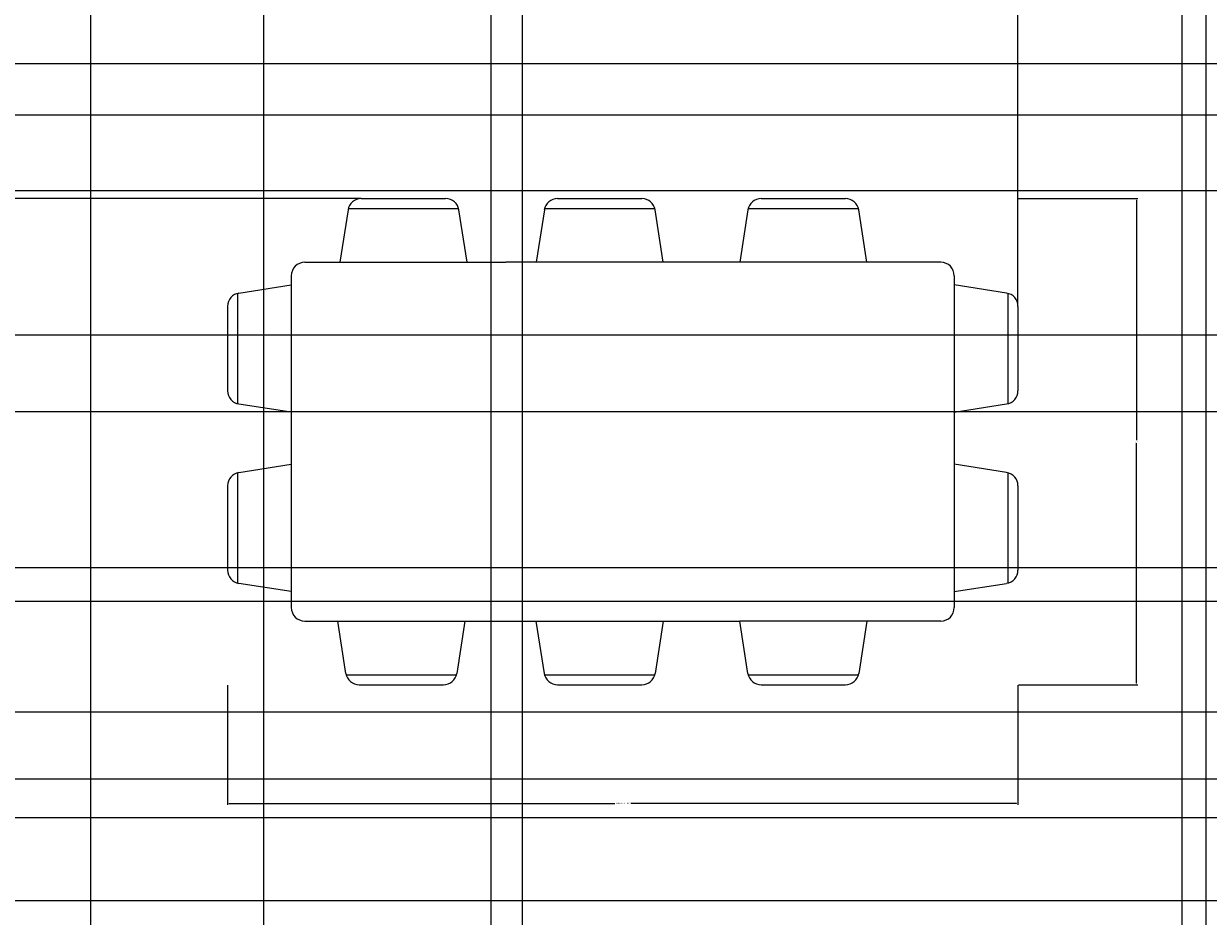
# Model space of a CAD drawing. Units: inches. Extents: x 1531 to 2263, y 2711 to 3216.
# Tile 8 of 12: x 1925 to 2076, y 2901 to 3015. Entities that reach past the tile are written whole.
import ezdxf

# ---------------------------------------------------------------- set-up
doc = ezdxf.new("R2010")
doc.units = ezdxf.units.IN
doc.layers.add('A-ANNO-DIMS', color=2, linetype='Continuous', lineweight=18)
doc.layers.add('A-FURN', color=8, linetype='Continuous', lineweight=18)
doc.styles.get("Standard").update_dxf_attribs({"font": 'arial.ttf'})
doc.dimstyles.get("Standard").update_dxf_attribs({"dimtxt": 0.18, "dimasz": 0.18, "dimexe": 0.18, "dimexo": 0.0625, "dimgap": 0.09, "dimtad": 0, "dimtih": 1, "dimtoh": 1, "dimdec": 4, "dimzin": 0, "dimdsep": 46, "dimtxsty": 'Standard', "dimcen": 0.09, "dimadec": 0, "dimazin": 0, "dimtfac": 1, "dimtdec": 4, "dimtofl": 0, "dimtmove": 0, "dimatfit": 3, "dimfxl": 1, "dimtolj": 1, "dimtzin": 0, "dimarcsym": 0})

# ---------------------------------------------------------------- blocks, each defined once
blk = doc.blocks.new('Dining Set - 36 x 72 in.')
for p, q in [((-27.5, -40.45), (-11.03, -40.45)), ((-25.56, -38.95), (-12.98, -38.95)), ((1.77, -40.45), (18.24, -40.45)), ((3.71, -38.95), (16.29, -38.95)), ((32.13, -40.45), (48.6, -40.45)), ((34.07, -38.95), (46.65, -38.95)), ((-27.53, -40.64), (-28.75, -48.45)), ((-9.78, -48.45), (-11.01, -40.64)), ((1.74, -40.64), (0.52, -48.45)), ((19.48, -48.45), (18.26, -40.64)), ((32.09, -40.64), (30.87, -48.45)), ((49.84, -48.45), (48.62, -40.64)), ((-34, -48.45), (-4, -48.45)), ((26.36, -48.45), (-4, -48.45)), ((60.87, -48.45), (26.36, -48.45)), ((49.84, -48.44), (30.87, -48.44)), ((-36, -50.45), (-36, -75.18)), ((62.87, -50.45), (62.87, -75.18)), ((-43.81, -53.04), (-36, -51.82)), ((70.68, -53.04), (62.87, -51.82)), ((-44, -53.07), (-44, -69.54)), ((70.87, -53.07), (70.87, -69.54)), ((-45.5, -55.01), (-45.5, -67.59)), ((72.37, -55.01), (72.37, -67.59)), ((-36, -70.79), (-43.81, -69.57)), ((62.87, -70.79), (70.68, -69.56)), ((-36, -75.18), (-36, -99.92)), ((62.87, -75.18), (62.87, -99.92)), ((-43.81, -79.77), (-36, -78.55)), ((70.68, -79.77), (62.87, -78.55)), ((-44, -79.81), (-44, -96.28)), ((70.87, -79.81), (70.87, -96.28)), ((-45.5, -81.75), (-45.5, -94.33)), ((72.37, -81.75), (72.37, -94.32)), ((-36, -97.52), (-43.81, -96.3)), ((62.87, -97.52), (70.68, -96.3)), ((-34, -101.92), (-4, -101.92)), ((-27.85, -109.73), (-29.07, -101.92)), ((-10.11, -101.92), (-11.33, -109.73)), ((-4, -101.92), (26.36, -101.92)), ((1.74, -109.73), (0.52, -101.92)), ((19.48, -101.92), (18.26, -109.73)), ((26.36, -101.92), (30.87, -101.92)), ((60.87, -101.92), (30.87, -101.92)), ((32.09, -109.73), (30.87, -101.92)), ((49.84, -101.92), (48.62, -109.73)), ((-27.82, -109.92), (-11.35, -109.92)), ((1.77, -109.92), (18.24, -109.92)), ((32.13, -109.92), (48.6, -109.92)), ((-25.88, -111.42), (-13.3, -111.42)), ((3.71, -111.42), (16.29, -111.42)), ((34.07, -111.42), (46.65, -111.42))]:
    blk.add_line(p, q)
for centre, start, end in [((-25.56, -40.95), 90, 171.1198), ((-12.98, -40.95), 8.881, 90), ((3.71, -40.95), 90, 171.1198), ((16.29, -40.95), 8.881, 90), ((34.07, -40.95), 90, 171.1198), ((46.65, -40.95), 8.881, 90), ((-34, -50.45), 90, 180), ((60.87, -50.45), 0, 90), ((-43.5, -55.01), 98.8806, 180), ((70.37, -55.01), 0, 81.1194), ((-43.5, -67.59), 180, 261.1194), ((70.37, -67.59), 278.8806, 0), ((-43.5, -81.75), 98.8806, 180), ((70.37, -81.75), 0, 81.1194), ((-43.5, -94.33), 180, 261.1194), ((70.37, -94.32), 278.8806, 0), ((-34, -99.92), 180, 270), ((60.87, -99.92), 270, 0), ((-25.88, -109.42), 188.8802, 270), ((-13.3, -109.42), 270, 351.1191), ((3.71, -109.42), 188.8802, 270), ((16.29, -109.42), 270, 351.1191), ((34.07, -109.42), 188.8802, 270), ((46.65, -109.42), 270, 351.1191)]:
    blk.add_arc(centre, 2, start, end)
blk = doc.blocks.new('*D52')
at = {"layer": 'A-ANNO-DIMS', "color": 0, "lineweight": -2, "transparency": 16777216}
for p, q in [((1951.34, 2930.78), (1951.34, 2915.57)), ((2052, 2930.78), (2052, 2915.57)), ((1951.52, 2915.75), (2000.65, 2915.75)), ((2051.82, 2915.75), (2002.69, 2915.75))]:
    blk.add_line(p, q, dxfattribs=at)
at = {"layer": 'A-ANNO-DIMS', "color": 0, "transparency": 16777216}
for points in [[(1951.52, 2915.78), (1951.52, 2915.72), (1951.34, 2915.75)], [(2051.82, 2915.78), (2051.82, 2915.72), (2052, 2915.75)]]:
    blk.add_solid(points, dxfattribs=at)
at = {"layer": 'Defpoints', "color": 0, "transparency": 16777216}
for p in [(1951.34, 2930.85), (2052, 2930.85), (2052, 2915.75)]:
    blk.add_point(p, dxfattribs=at)
at = {"layer": 'A-ANNO-DIMS', "color": 0, "transparency": 16777216, "insert": (2001.67, 2915.75), "char_height": 0.18, "attachment_point": 5}
blk.add_mtext('\\A1;DINING SET 101', dxfattribs=at)
blk = doc.blocks.new('*D53')
at = {"layer": 'A-ANNO-DIMS', "color": 0, "lineweight": -2, "transparency": 16777216}
for p, q in [((2052.06, 2992.73), (2067.28, 2992.73)), ((2067.1, 2992.55), (2067.1, 2961.97)), ((2067.1, 2931.03), (2067.1, 2961.61)), ((2052.06, 2930.85), (2067.28, 2930.85))]:
    blk.add_line(p, q, dxfattribs=at)
at = {"layer": 'A-ANNO-DIMS', "color": 0, "transparency": 16777216}
for points in [[(2067.07, 2992.55), (2067.13, 2992.55), (2067.1, 2992.73)], [(2067.07, 2931.03), (2067.13, 2931.03), (2067.1, 2930.85)]]:
    blk.add_solid(points, dxfattribs=at)
at = {"layer": 'Defpoints', "color": 0, "transparency": 16777216}
for p in [(2052, 2992.73), (2067.1, 2992.73), (2052, 2930.85)]:
    blk.add_point(p, dxfattribs=at)
at = {"layer": 'A-ANNO-DIMS', "color": 0, "transparency": 16777216, "insert": (2067.1, 2961.79), "char_height": 0.18, "attachment_point": 5}
blk.add_mtext('\\A1;62', dxfattribs=at)
blk = doc.blocks.new('*D60')
at = {"layer": 'A-ANNO-DIMS', "color": 0, "lineweight": -2, "transparency": 16777216}
for p, q in [((1899.91, 3097.79), (1899.91, 2711.06)), ((1955.91, 3097.81), (1955.91, 2711.06)), ((1900.09, 2711.24), (1927.69, 2711.24)), ((1955.73, 2711.24), (1928.13, 2711.24))]:
    blk.add_line(p, q, dxfattribs=at)
at = {"layer": 'A-ANNO-DIMS', "color": 0, "transparency": 16777216}
for points in [[(1900.09, 2711.27), (1900.09, 2711.21), (1899.91, 2711.24)], [(1955.73, 2711.27), (1955.73, 2711.21), (1955.91, 2711.24)]]:
    blk.add_solid(points, dxfattribs=at)
at = {"layer": 'Defpoints', "color": 0, "transparency": 16777216}
for p in [(1899.91, 3097.85), (1955.91, 3097.88), (1955.91, 2711.24)]:
    blk.add_point(p, dxfattribs=at)
at = {"layer": 'A-ANNO-DIMS', "color": 0, "transparency": 16777216, "insert": (1927.91, 2711.24), "char_height": 0.18, "attachment_point": 5}
blk.add_mtext('\\A1;56', dxfattribs=at)
blk = doc.blocks.new('*D71')
at = {"layer": 'A-ANNO-DIMS', "color": 0, "lineweight": -2, "transparency": 16777216}
for p, q in [((1933.91, 2891.93), (1933.91, 3216.47)), ((1984.91, 2891.95), (1984.91, 3216.47)), ((1934.09, 3216.29), (1959.21, 3216.29)), ((1984.73, 3216.29), (1959.61, 3216.29))]:
    blk.add_line(p, q, dxfattribs=at)
at = {"layer": 'A-ANNO-DIMS', "color": 0, "transparency": 16777216}
for points in [[(1934.09, 3216.32), (1934.09, 3216.26), (1933.91, 3216.29)], [(1984.73, 3216.32), (1984.73, 3216.26), (1984.91, 3216.29)]]:
    blk.add_solid(points, dxfattribs=at)
at = {"layer": 'Defpoints', "color": 0, "transparency": 16777216}
for p in [(1984.91, 3216.29), (1933.91, 2891.87), (1984.91, 2891.89)]:
    blk.add_point(p, dxfattribs=at)
at = {"layer": 'A-ANNO-DIMS', "color": 0, "transparency": 16777216, "insert": (1959.41, 3216.29), "char_height": 0.18, "attachment_point": 5}
blk.add_mtext('\\A1;51', dxfattribs=at)
blk = doc.blocks.new('*D77')
at = {"layer": 'A-ANNO-DIMS', "color": 0, "lineweight": -2, "transparency": 16777216}
for p, q in [((2094.81, 2975.33), (1531.04, 2975.33)), ((1531.22, 2975.15), (1531.22, 2939.52)), ((1531.22, 2903.53), (1531.22, 2939.16)), ((2094.81, 2903.35), (1531.04, 2903.35))]:
    blk.add_line(p, q, dxfattribs=at)
at = {"layer": 'A-ANNO-DIMS', "color": 0, "transparency": 16777216}
for points in [[(1531.19, 2975.15), (1531.25, 2975.15), (1531.22, 2975.33)], [(1531.19, 2903.53), (1531.25, 2903.53), (1531.22, 2903.35)]]:
    blk.add_solid(points, dxfattribs=at)
at = {"layer": 'Defpoints', "color": 0, "transparency": 16777216}
for p in [(2094.87, 2975.33), (1531.22, 2903.35), (2094.87, 2903.35)]:
    blk.add_point(p, dxfattribs=at)
at = {"layer": 'A-ANNO-DIMS', "color": 0, "transparency": 16777216, "insert": (1531.22, 2939.34), "char_height": 0.18, "attachment_point": 5}
blk.add_mtext('\\A1;71.98', dxfattribs=at)
blk = doc.blocks.new('*D79')
at = {"layer": 'A-ANNO-DIMS', "color": 0, "lineweight": -2, "transparency": 16777216}
for p, q in [((1988.91, 2807.93), (1988.91, 3216.47)), ((2072.91, 2807.93), (2072.91, 3216.47)), ((1989.09, 3216.29), (2030.69, 3216.29)), ((2072.73, 3216.29), (2031.13, 3216.29))]:
    blk.add_line(p, q, dxfattribs=at)
at = {"layer": 'A-ANNO-DIMS', "color": 0, "transparency": 16777216}
for points in [[(1989.09, 3216.32), (1989.09, 3216.26), (1988.91, 3216.29)], [(2072.73, 3216.32), (2072.73, 3216.26), (2072.91, 3216.29)]]:
    blk.add_solid(points, dxfattribs=at)
at = {"layer": 'Defpoints', "color": 0, "transparency": 16777216}
for p in [(2072.91, 3216.29), (1988.91, 2807.86), (2072.91, 2807.86)]:
    blk.add_point(p, dxfattribs=at)
at = {"layer": 'A-ANNO-DIMS', "color": 0, "transparency": 16777216, "insert": (2030.91, 3216.29), "char_height": 0.18, "attachment_point": 5}
blk.add_mtext('\\A1;84', dxfattribs=at)
blk = doc.blocks.new('*D99')
at = {"layer": 'A-ANNO-DIMS', "color": 0, "lineweight": -2, "transparency": 16777216}
for p, q in [((1894.62, 3003.38), (2262.37, 3003.38)), ((2262.19, 3003.2), (2262.19, 2965.56)), ((2262.19, 2927.56), (2262.19, 2965.19)), ((1894.62, 2927.38), (2262.37, 2927.38))]:
    blk.add_line(p, q, dxfattribs=at)
at = {"layer": 'A-ANNO-DIMS', "color": 0, "transparency": 16777216}
for points in [[(2262.16, 3003.2), (2262.22, 3003.2), (2262.19, 3003.38)], [(2262.16, 2927.56), (2262.22, 2927.56), (2262.19, 2927.38)]]:
    blk.add_solid(points, dxfattribs=at)
at = {"layer": 'Defpoints', "color": 0, "transparency": 16777216}
for p in [(1894.55, 3003.38), (1894.55, 2927.38), (2262.19, 2927.38)]:
    blk.add_point(p, dxfattribs=at)
at = {"layer": 'A-ANNO-DIMS', "color": 0, "transparency": 16777216, "insert": (2262.19, 2965.38), "char_height": 0.18, "attachment_point": 5}
blk.add_mtext('\\A1;76', dxfattribs=at)
blk = doc.blocks.new('*D101')
at = {"layer": 'A-ANNO-DIMS', "color": 0, "lineweight": -2, "transparency": 16777216}
for p, q in [((2228.85, 2918.81), (1531.04, 2918.81)), ((1531.22, 2918.63), (1531.22, 2897.08)), ((1531.22, 2875.18), (1531.22, 2896.72)), ((2228.85, 2875), (1531.04, 2875))]:
    blk.add_line(p, q, dxfattribs=at)
at = {"layer": 'A-ANNO-DIMS', "color": 0, "transparency": 16777216}
for points in [[(1531.19, 2918.63), (1531.25, 2918.63), (1531.22, 2918.81)], [(1531.19, 2875.18), (1531.25, 2875.18), (1531.22, 2875)]]:
    blk.add_solid(points, dxfattribs=at)
at = {"layer": 'Defpoints', "color": 0, "transparency": 16777216}
for p in [(2228.91, 2918.81), (1531.22, 2875), (2228.91, 2875)]:
    blk.add_point(p, dxfattribs=at)
at = {"layer": 'A-ANNO-DIMS', "color": 0, "transparency": 16777216, "insert": (1531.22, 2896.9), "char_height": 0.18, "attachment_point": 5}
blk.add_mtext('\\A1;43.81', dxfattribs=at)
blk = doc.blocks.new('*D112')
at = {"layer": 'A-ANNO-DIMS', "color": 0, "lineweight": -2, "transparency": 16777216}
for p, q in [((1721.97, 3009.94), (2262.37, 3009.94)), ((2262.19, 3009.76), (2262.19, 2962.12)), ((2262.19, 2914.12), (2262.19, 2961.76)), ((1721.97, 2913.94), (2262.37, 2913.94))]:
    blk.add_line(p, q, dxfattribs=at)
at = {"layer": 'A-ANNO-DIMS', "color": 0, "transparency": 16777216}
for points in [[(2262.16, 3009.76), (2262.22, 3009.76), (2262.19, 3009.94)], [(2262.16, 2914.12), (2262.22, 2914.12), (2262.19, 2913.94)]]:
    blk.add_solid(points, dxfattribs=at)
at = {"layer": 'Defpoints', "color": 0, "transparency": 16777216}
for p in [(1721.91, 3009.94), (1721.91, 2913.94), (2262.19, 2913.94)]:
    blk.add_point(p, dxfattribs=at)
at = {"layer": 'A-ANNO-DIMS', "color": 0, "transparency": 16777216, "insert": (2262.19, 2961.94), "char_height": 0.18, "attachment_point": 5}
blk.add_mtext('\\A1;96', dxfattribs=at)
blk = doc.blocks.new('*D114')
at = {"layer": 'A-ANNO-DIMS', "color": 0, "lineweight": -2, "transparency": 16777216}
for p, q in [((1577.97, 2913.94), (2262.37, 2913.94)), ((2262.19, 2913.76), (2262.19, 2904.99)), ((2262.19, 2895.86), (2262.19, 2904.63)), ((1577.97, 2895.68), (2262.37, 2895.68))]:
    blk.add_line(p, q, dxfattribs=at)
at = {"layer": 'A-ANNO-DIMS', "color": 0, "transparency": 16777216}
for points in [[(2262.16, 2913.76), (2262.22, 2913.76), (2262.19, 2913.94)], [(2262.16, 2895.86), (2262.22, 2895.86), (2262.19, 2895.68)]]:
    blk.add_solid(points, dxfattribs=at)
at = {"layer": 'Defpoints', "color": 0, "transparency": 16777216}
for p in [(1577.91, 2913.94), (1577.91, 2895.68), (2262.19, 2895.68)]:
    blk.add_point(p, dxfattribs=at)
at = {"layer": 'A-ANNO-DIMS', "color": 0, "transparency": 16777216, "insert": (2262.19, 2904.81), "char_height": 0.18, "attachment_point": 5}
blk.add_mtext('\\A1;18.26', dxfattribs=at)
blk = doc.blocks.new('*D116')
at = {"layer": 'A-ANNO-DIMS', "color": 0, "lineweight": -2, "transparency": 16777216}
for p, q in [((1899.97, 3025.85), (2262.37, 3025.85)), ((2262.19, 3025.67), (2262.19, 3014.79)), ((2262.19, 3003.56), (2262.19, 3014.43)), ((1894.62, 3003.38), (2262.37, 3003.38))]:
    blk.add_line(p, q, dxfattribs=at)
at = {"layer": 'A-ANNO-DIMS', "color": 0, "transparency": 16777216}
for points in [[(2262.16, 3025.67), (2262.22, 3025.67), (2262.19, 3025.85)], [(2262.16, 3003.56), (2262.22, 3003.56), (2262.19, 3003.38)]]:
    blk.add_solid(points, dxfattribs=at)
at = {"layer": 'Defpoints', "color": 0, "transparency": 16777216}
for p in [(1899.91, 3025.85), (1894.55, 3003.38), (2262.19, 3003.38)]:
    blk.add_point(p, dxfattribs=at)
at = {"layer": 'A-ANNO-DIMS', "color": 0, "transparency": 16777216, "insert": (2262.19, 3014.61), "char_height": 0.18, "attachment_point": 5}
blk.add_mtext('\\A1;22.47', dxfattribs=at)
blk = doc.blocks.new('*D118')
at = {"layer": 'A-ANNO-DIMS', "color": 0, "lineweight": -2, "transparency": 16777216}
for p, q in [((1851.5, 2965.63), (2262.37, 2965.63)), ((2262.19, 2965.45), (2262.19, 2953.74)), ((2262.19, 2941.67), (2262.19, 2953.38)), ((1851.5, 2941.49), (2262.37, 2941.49))]:
    blk.add_line(p, q, dxfattribs=at)
at = {"layer": 'A-ANNO-DIMS', "color": 0, "transparency": 16777216}
for points in [[(2262.16, 2965.45), (2262.22, 2965.45), (2262.19, 2965.63)], [(2262.16, 2941.67), (2262.22, 2941.67), (2262.19, 2941.49)]]:
    blk.add_solid(points, dxfattribs=at)
at = {"layer": 'Defpoints', "color": 0, "transparency": 16777216}
for p in [(1851.44, 2965.63), (1851.44, 2941.49), (2262.19, 2941.49)]:
    blk.add_point(p, dxfattribs=at)
at = {"layer": 'A-ANNO-DIMS', "color": 0, "transparency": 16777216, "insert": (2262.19, 2953.56), "char_height": 0.18, "attachment_point": 5}
blk.add_mtext('\\A1;24.14', dxfattribs=at)
blk = doc.blocks.new('*D120')
at = {"layer": 'A-ANNO-DIMS', "color": 0, "lineweight": -2, "transparency": 16777216}
for p, q in [((1797.97, 2993.76), (2262.37, 2993.76)), ((2262.19, 2993.58), (2262.19, 2969.95)), ((2262.19, 2945.94), (2262.19, 2969.58)), ((1797.97, 2945.76), (2262.37, 2945.76))]:
    blk.add_line(p, q, dxfattribs=at)
at = {"layer": 'A-ANNO-DIMS', "color": 0, "transparency": 16777216}
for points in [[(2262.16, 2993.58), (2262.22, 2993.58), (2262.19, 2993.76)], [(2262.16, 2945.94), (2262.22, 2945.94), (2262.19, 2945.76)]]:
    blk.add_solid(points, dxfattribs=at)
at = {"layer": 'Defpoints', "color": 0, "transparency": 16777216}
for p in [(1797.91, 2993.76), (2262.19, 2993.76), (1797.91, 2945.76)]:
    blk.add_point(p, dxfattribs=at)
at = {"layer": 'A-ANNO-DIMS', "color": 0, "transparency": 16777216, "insert": (2262.19, 2969.76), "char_height": 0.18, "attachment_point": 5}
blk.add_mtext('\\A1;48', dxfattribs=at)
blk = doc.blocks.new('*D121')
at = {"layer": 'A-ANNO-DIMS', "color": 0, "lineweight": -2, "transparency": 16777216}
for p, q in [((2052, 2979.08), (2052, 3216.47)), ((2094.87, 2979.39), (2094.87, 3216.47)), ((2052.18, 3216.29), (2073.04, 3216.29)), ((2094.69, 3216.29), (2073.83, 3216.29))]:
    blk.add_line(p, q, dxfattribs=at)
at = {"layer": 'A-ANNO-DIMS', "color": 0, "transparency": 16777216}
for points in [[(2052.18, 3216.32), (2052.18, 3216.26), (2052, 3216.29)], [(2094.69, 3216.32), (2094.69, 3216.26), (2094.87, 3216.29)]]:
    blk.add_solid(points, dxfattribs=at)
at = {"layer": 'Defpoints', "color": 0, "transparency": 16777216}
for p in [(2094.87, 3216.29), (2052, 2979.01), (2094.87, 2979.33)]:
    blk.add_point(p, dxfattribs=at)
at = {"layer": 'A-ANNO-DIMS', "color": 0, "transparency": 16777216, "insert": (2073.43, 3216.29), "char_height": 0.18, "attachment_point": 5}
blk.add_mtext('\\A1;42.87', dxfattribs=at)
blk = doc.blocks.new('*D122')
at = {"layer": 'A-ANNO-DIMS', "color": 0, "lineweight": -2, "transparency": 16777216}
for p, q in [((1955.85, 3025.88), (1531.04, 3025.88)), ((1531.22, 3025.7), (1531.22, 3009.49)), ((1531.22, 2992.91), (1531.22, 3009.12)), ((1968.31, 2992.73), (1531.04, 2992.73))]:
    blk.add_line(p, q, dxfattribs=at)
at = {"layer": 'A-ANNO-DIMS', "color": 0, "transparency": 16777216}
for points in [[(1531.19, 3025.7), (1531.25, 3025.7), (1531.22, 3025.88)], [(1531.19, 2992.91), (1531.25, 2992.91), (1531.22, 2992.73)]]:
    blk.add_solid(points, dxfattribs=at)
at = {"layer": 'Defpoints', "color": 0, "transparency": 16777216}
for p in [(1531.22, 3025.88), (1955.91, 3025.88), (1968.37, 2992.73)]:
    blk.add_point(p, dxfattribs=at)
at = {"layer": 'A-ANNO-DIMS', "color": 0, "transparency": 16777216, "insert": (1531.22, 3009.3), "char_height": 0.18, "attachment_point": 5}
blk.add_mtext('\\A1;33.146', dxfattribs=at)
blk = doc.blocks.new('*D130')
at = {"layer": 'A-ANNO-DIMS', "color": 0, "lineweight": -2, "transparency": 16777216}
for p, q in [((2075.91, 3029.88), (2075.91, 2711.06)), ((2079.91, 3025.88), (2079.91, 2711.06)), ((2076.09, 2711.24), (2077.76, 2711.24)), ((2079.73, 2711.24), (2078.06, 2711.24))]:
    blk.add_line(p, q, dxfattribs=at)
at = {"layer": 'A-ANNO-DIMS', "color": 0, "transparency": 16777216}
for points in [[(2076.09, 2711.27), (2076.09, 2711.21), (2075.91, 2711.24)], [(2079.73, 2711.27), (2079.73, 2711.21), (2079.91, 2711.24)]]:
    blk.add_solid(points, dxfattribs=at)
at = {"layer": 'Defpoints', "color": 0, "transparency": 16777216}
for p in [(2075.91, 3029.94), (2079.91, 3025.94), (2075.91, 2711.24)]:
    blk.add_point(p, dxfattribs=at)
at = {"layer": 'A-ANNO-DIMS', "color": 0, "transparency": 16777216, "insert": (2077.91, 2711.24), "char_height": 0.18, "attachment_point": 5}
blk.add_mtext('\\A1;4', dxfattribs=at)

msp = doc.modelspace()

# ---------------------------------------------------------------- block references
at = {"layer": 'A-FURN', "xscale": 0.8539401252777441, "yscale": 0.8539401252777441, "zscale": 0.8539401252777441}
msp.add_blockref('Dining Set - 36 x 72 in.', (1990.1969, 3025.9901), dxfattribs=at)

# ---------------------------------------------------------------- dimensions: what is measured, and where the dimension line sits
at = {"layer": 'A-ANNO-DIMS'}
for base, p1, p2, override, picture, middle in [((1984.9101, 3216.295), (1933.9101, 2891.8657), (1984.9101, 2891.8924), {"dimdec": 0, "dimlfac": 1, "dimrnd": 0, "dimzin": 0, "dimdsep": 46, "dimlunit": 2}, '*D71', (1959.4101, 3216.295)), ((2072.9101, 3216.295), (1988.9101, 2807.8631), (2072.9101, 2807.8631), {"dimdec": 0, "dimlfac": 1, "dimrnd": 0, "dimzin": 0, "dimdsep": 46, "dimlunit": 2}, '*D79', (2030.9101, 3216.295)), ((2094.8704, 3216.295), (2051.9983, 2979.0128), (2094.8704, 2979.3315), {"dimdec": 2, "dimlfac": 1, "dimrnd": 0, "dimzin": 0, "dimdsep": 46, "dimlunit": 2}, '*D121', (2073.4343, 3216.295)), ((1955.9101, 2711.2407), (1899.9101, 3097.8479), (1955.9101, 3097.8772), {"dimdec": 0, "dimlfac": 1, "dimrnd": 0, "dimzin": 0, "dimdsep": 46, "dimlunit": 2}, '*D60', (1927.9101, 2711.2407)), ((2075.9101, 2711.2407), (2079.9101, 3025.9421), (2075.9101, 3029.94), {"dimdec": 0, "dimlfac": 1, "dimrnd": 0, "dimzin": 0, "dimdsep": 46, "dimlunit": 2}, '*D130', (2077.9101, 2711.2407))]:
    dim = msp.add_linear_dim(base=base, p1=p1, p2=p2, dimstyle='Standard', override=override, dxfattribs=at)
    dim.commit()
    dim.dimension.update_dxf_attribs({"geometry": picture, "text_midpoint": middle})
for base, p1, p2, override, picture, middle in [((1531.2212, 3025.8772), (1968.3722, 2992.7314), (1955.9101, 3025.8772), {"dimdec": 3, "dimlfac": 1, "dimrnd": 0, "dimzin": 0, "dimdsep": 46, "dimlunit": 2}, '*D122', (1531.2212, 3009.3043)), ((2262.1851, 3003.376), (1899.9101, 3025.8479), (1894.5532, 3003.376), {"dimdec": 2, "dimlfac": 1, "dimrnd": 0, "dimzin": 0, "dimdsep": 46, "dimlunit": 2}, '*D116', (2262.1851, 3014.6119)), ((2262.1851, 2913.9378), (1721.9111, 3009.9378), (1721.9111, 2913.9378), {"dimdec": 0, "dimlfac": 1, "dimrnd": 0, "dimzin": 0, "dimdsep": 46, "dimlunit": 2}, '*D112', (2262.1851, 2961.9378)), ((2262.1851, 2927.376), (1894.5532, 3003.376), (1894.5532, 2927.376), {"dimdec": 0, "dimlfac": 1, "dimrnd": 0, "dimzin": 0, "dimdsep": 46, "dimlunit": 2}, '*D99', (2262.1851, 2965.376)), ((2262.1851, 2993.7637), (1797.9101, 2945.7637), (1797.9101, 2993.7637), {"dimdec": 0, "dimlfac": 1, "dimrnd": 0, "dimzin": 0, "dimdsep": 46, "dimlunit": 2}, '*D120', (2262.1851, 2969.7637)), ((2067.0966, 2992.7314), (2051.9983, 2930.8451), (2051.9983, 2992.7314), {"dimdec": 0, "dimlfac": 1, "dimrnd": 0, "dimzin": 0, "dimdsep": 46, "dimlunit": 2}, '*D53', (2067.0966, 2961.7883)), ((1531.2212, 2903.3482), (2094.8725, 2975.3315), (2094.8725, 2903.3482), {"dimdec": 2, "dimlfac": 1, "dimrnd": 0, "dimzin": 0, "dimdsep": 46, "dimlunit": 2}, '*D77', (1531.2212, 2939.3398)), ((2262.1851, 2941.4913), (1851.4391, 2965.6329), (1851.4391, 2941.4913), {"dimdec": 2, "dimlfac": 1, "dimrnd": 0, "dimzin": 0, "dimdsep": 46, "dimlunit": 2}, '*D118', (2262.1851, 2953.5621)), ((1531.2212, 2874.9957), (2228.9101, 2918.8056), (2228.9101, 2874.9957), {"dimdec": 2, "dimlfac": 1, "dimrnd": 0, "dimzin": 0, "dimdsep": 46, "dimlunit": 2}, '*D101', (1531.2212, 2896.9007)), ((2262.1851, 2895.6796), (1577.9111, 2913.9378), (1577.9111, 2895.6796), {"dimdec": 2, "dimlfac": 1, "dimrnd": 0, "dimzin": 0, "dimdsep": 46, "dimlunit": 2}, '*D114', (2262.1851, 2904.8087))]:
    dim = msp.add_linear_dim(base=base, p1=p1, p2=p2, angle=90, dimstyle='Standard', override=override, dxfattribs=at)
    dim.commit()
    dim.dimension.update_dxf_attribs({"geometry": picture, "text_midpoint": middle})
dim = msp.add_linear_dim(base=(2051.9983, 2915.7467), p1=(1951.3426, 2930.8451), p2=(2051.9983, 2930.8451), text='DINING SET <>', dimstyle='Standard', override={"dimdec": 0, "dimlfac": 1, "dimrnd": 0, "dimzin": 0, "dimdsep": 46, "dimlunit": 2}, dxfattribs=at)
dim.commit()
dim.dimension.update_dxf_attribs({"geometry": '*D52', "text_midpoint": (2001.6704, 2915.7467)})

doc.saveas('drawing.dxf')
